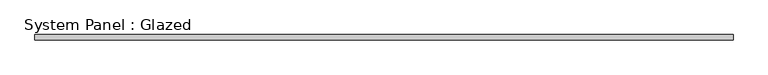
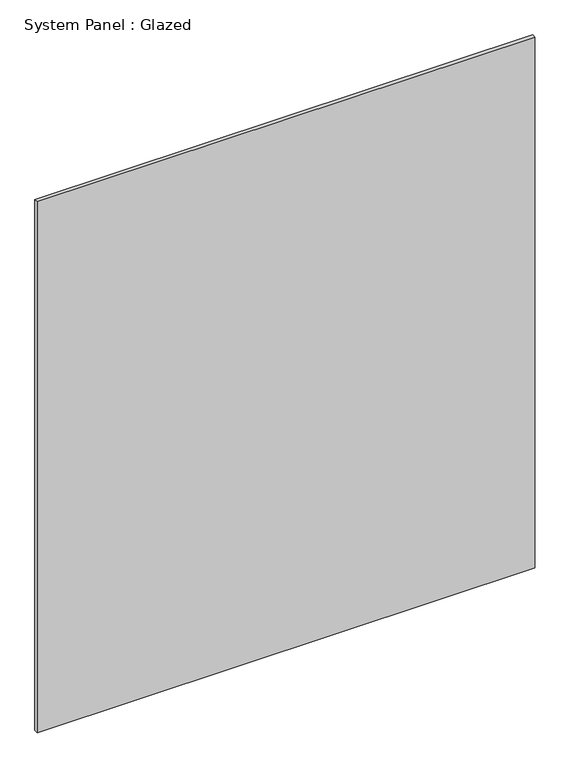
"""IFC4 building model written with IfcOpenShell, lengths in millimetres: plate geometry, System Panel : Glazed."""

from ifc_helpers import new_model, si_unit, origin, origin_with_axes, place, context, project, spatial, polyline, outline, extrude, source, transform, mapped, element, save


def system_panel_glazed_8a9794be(model_context):
    return source(origin(), model_context, "Body", "SweptSolid", [
        extrude(outline(polyline([(1700.0503139, 19.05), (-1700.0503139, 19.05), (-1700.0503139, 44.45), (1700.0503139, 44.45), (1700.0503139, 19.05)])), origin_with_axes(), (0.0, 0.0, 1.0), 3835.4),
    ])


if __name__ == "__main__":
    model = new_model("IFC4")
    model_context = context("Model", 3, world=origin())
    ifc_project = project(units=[si_unit("LENGTHUNIT", "METRE", prefix="MILLI")], contexts=[model_context])
    site = spatial("IfcSite", under=ifc_project)
    building = spatial("IfcBuilding", under=site)
    placement = place(None, origin())
    system_panel_glazed_shape = system_panel_glazed_8a9794be(model_context)
    element("IfcPlate", 1, ObjectType="System Panel : Glazed", at=placement, inside=building, context=model_context, shape_type="MappedRepresentation", body=[
        mapped(system_panel_glazed_shape, transform((0.0, 0.0, 0.0), x_axis=(1.0, 0.0, 0.0), y_axis=(0.0, 1.0, 0.0), z_axis=(0.0, 0.0, 1.0))),
    ])
    save(model, "model.ifc")

# Revit data of these elements
# Type "System Panel : Glazed"
#   Construction Type Id = "GSP4R"
#   Analytic Construction = "1/8 in Pilkington single glazing"
#   Visual Light Transmittance = 0.9
#   Solar Heat Gain Coefficient = 0.86
#   Heat Transfer Coefficient (U) = 1.18115 BTU/(h·ft²·°F)
# Element 1 (IfcPlate, "System Panel : Glazed")
#   Materials on its faces: "Glass"
# Materials
#   "Glass": class "Glass", colour RGB 0 128 192, transparency 0.75, Description = "Soda Lime Glass", Cost = 0
